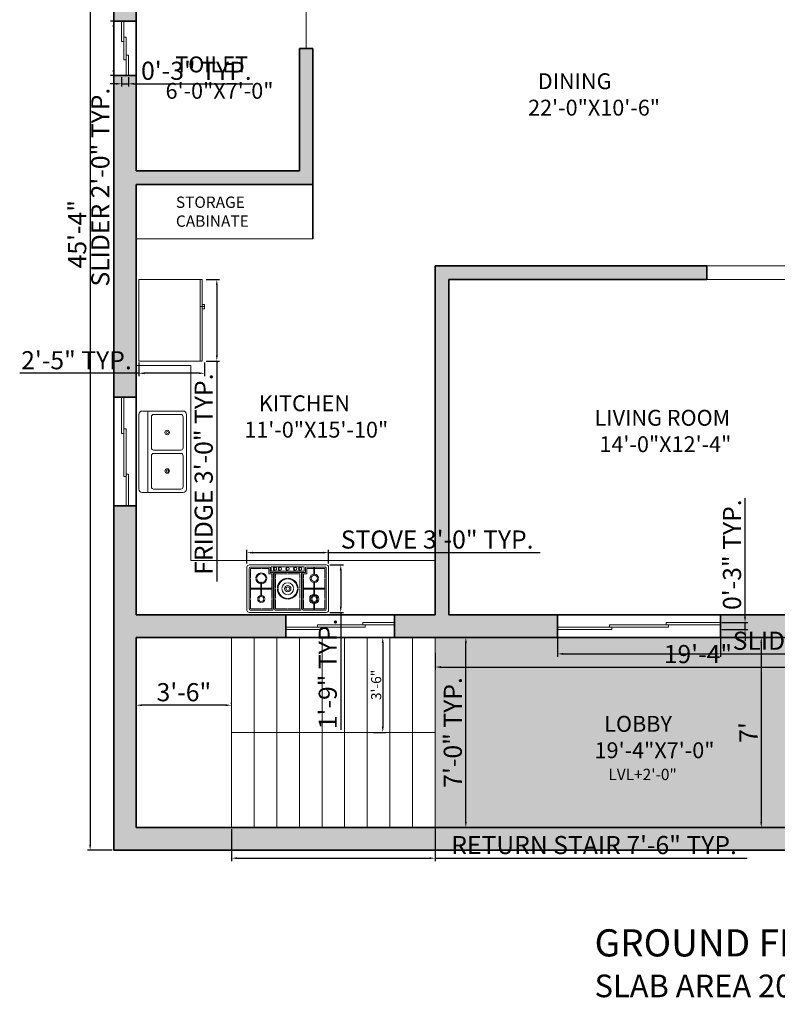
# Model space of a CAD drawing. Units: inches. Extents: x 3491 to 6898, y 1360 to 2019.
# Tile 1 of 9: x 3491 to 3825, y 1360 to 1795. Entities that reach past the tile are written whole.
import ezdxf

# ---------------------------------------------------------------- set-up
doc = ezdxf.new("R2010")
doc.units = ezdxf.units.IN
for name, color, linetype, lineweight in [('A-ANNO-DIMS', 2, 'Continuous', 18), ('A-ANNO-TEXT', 7, 'Continuous', 18), ('A-ANNO-TITL', 7, 'Continuous', 30), ('A-AREA-IDEN', 7, 'Continuous', 18), ('A-DOOR', 4, 'Continuous', 18), ('A-EQPM', 8, 'Continuous', 18), ('A-FLOR-CASE', 8, 'Continuous', 18), ('A-FLOR-FIXT', 8, 'Continuous', 18), ('A-FLOR-PATT', 252, 'Continuous', 13), ('A-FLOR-STRS', 7, 'Continuous', 18), ('A-GLAZ', 5, 'Continuous', 18), ('A-WALL', 7, 'Continuous', 35), ('A-WALL-PATT', 8, 'Continuous', 13)]:
    doc.layers.add(name, color=color, linetype=linetype, lineweight=lineweight)
doc.layers.add('A-WALL-OPEN', color=251, linetype='Continuous', lineweight=13, true_color=0x636466)
doc.styles.get("Standard").update_dxf_attribs({"font": 'arial.ttf'})
doc.dimstyles.new('ISO-25', dxfattribs={"dimtxt": 8, "dimasz": 2.5, "dimexe": 1.25, "dimexo": 0.625, "dimtad": 1, "dimdec": 1, "dimlunit": 3, "dimtxsty": 'Standard', "dimcen": 2.5, "dimclrt": 1, "dimadec": 0, "dimazin": 0, "dimtfac": 1, "dimtdec": 1, "dimtmove": 0, "dimatfit": 3, "dimfxl": 1, "dimarcsym": 0})

# ---------------------------------------------------------------- blocks, each defined once
blk = doc.blocks.new('*D4')
at = {"layer": 'A-ANNO-DIMS', "color": 0, "lineweight": -2, "transparency": 16777216}
for p, q in [((3531.51, 1972.37), (3520.5, 1972.37)), ((3521.75, 1969.87), (3521.75, 1430.87)), ((3531.51, 1428.37), (3520.5, 1428.37))]:
    blk.add_line(p, q, dxfattribs=at)
at = {"layer": 'A-ANNO-DIMS', "color": 0, "transparency": 16777216}
for points in [[(3521.33, 1969.87), (3522.17, 1969.87), (3521.75, 1972.37)], [(3521.33, 1430.87), (3522.17, 1430.87), (3521.75, 1428.37)]]:
    blk.add_solid(points, dxfattribs=at)
at = {"layer": 'Defpoints', "color": 0, "transparency": 16777216}
for p in [(3532.13, 1972.37), (3521.75, 1428.37), (3532.13, 1428.37)]:
    blk.add_point(p, dxfattribs=at)
at = {"layer": 'A-ANNO-DIMS', "color": 0, "transparency": 16777216, "insert": (3517.06, 1700.37), "char_height": 8, "attachment_point": 5, "rotation": 90}
blk.add_mtext('45\'-4"', dxfattribs=at)
blk = doc.blocks.new('*D5')
at = {"layer": 'A-ANNO-DIMS', "color": 0, "lineweight": -2, "transparency": 16777216}
for p, q in [((3542.13, 1493.03), (3542.13, 1493.65)), ((3581.63, 1492.4), (3544.63, 1492.4)), ((3584.13, 1493.03), (3584.13, 1493.65))]:
    blk.add_line(p, q, dxfattribs=at)
at = {"layer": 'A-ANNO-DIMS', "color": 0, "transparency": 16777216}
for points in [[(3544.63, 1492.82), (3544.63, 1491.99), (3542.13, 1492.4)], [(3581.63, 1492.82), (3581.63, 1491.99), (3584.13, 1492.4)]]:
    blk.add_solid(points, dxfattribs=at)
at = {"layer": 'Defpoints', "color": 0, "transparency": 16777216}
for p in [(3542.13, 1492.4), (3542.13, 1492.4), (3584.13, 1492.4)]:
    blk.add_point(p, dxfattribs=at)
at = {"layer": 'A-ANNO-DIMS', "color": 0, "transparency": 16777216, "insert": (3563.13, 1497.12), "char_height": 8, "attachment_point": 5}
blk.add_mtext('3\'-6"', dxfattribs=at)
blk = doc.blocks.new('*D6')
at = {"layer": 'A-ANNO-DIMS', "color": 0, "lineweight": -2, "transparency": 16777216}
for p, q in [((3646.84, 1522.37), (3652.19, 1522.37)), ((3650.94, 1519.87), (3650.94, 1482.87)), ((3646.84, 1480.37), (3652.19, 1480.37))]:
    blk.add_line(p, q, dxfattribs=at)
at = {"layer": 'A-ANNO-DIMS', "color": 0, "transparency": 16777216}
for points in [[(3650.52, 1519.87), (3651.36, 1519.87), (3650.94, 1522.37)], [(3650.52, 1482.87), (3651.36, 1482.87), (3650.94, 1480.37)]]:
    blk.add_solid(points, dxfattribs=at)
at = {"layer": 'Defpoints', "color": 0, "transparency": 16777216}
for p in [(3646.22, 1522.37), (3646.22, 1480.37), (3650.94, 1480.37)]:
    blk.add_point(p, dxfattribs=at)
at = {"layer": 'A-ANNO-DIMS', "color": 0, "transparency": 16777216, "insert": (3648.04, 1501.37), "char_height": 8, "attachment_point": 5, "rotation": 90}
blk.add_mtext('{\\H0.55556x;3\'-6"}', dxfattribs=at)
blk = doc.blocks.new('*D7')
at = {"layer": 'A-ANNO-DIMS', "color": 0, "lineweight": -2, "transparency": 16777216}
for p, q in [((3818.73, 1522.37), (3819.35, 1522.37)), ((3818.1, 1519.87), (3818.1, 1440.87)), ((3818.73, 1438.37), (3819.35, 1438.37))]:
    blk.add_line(p, q, dxfattribs=at)
at = {"layer": 'A-ANNO-DIMS', "color": 0, "transparency": 16777216}
for points in [[(3817.69, 1519.87), (3818.52, 1519.87), (3818.1, 1522.37)], [(3817.69, 1440.87), (3818.52, 1440.87), (3818.1, 1438.37)]]:
    blk.add_solid(points, dxfattribs=at)
at = {"layer": 'Defpoints', "color": 0, "transparency": 16777216}
for p in [(3818.1, 1522.37), (3818.1, 1438.37), (3818.1, 1438.37)]:
    blk.add_point(p, dxfattribs=at)
at = {"layer": 'A-ANNO-DIMS', "color": 0, "transparency": 16777216, "insert": (3813.48, 1480.37), "char_height": 8, "attachment_point": 5, "rotation": 90}
blk.add_mtext("7'", dxfattribs=at)
blk = doc.blocks.new('*D8')
at = {"layer": 'A-ANNO-DIMS', "color": 0, "lineweight": -2, "transparency": 16777216}
for p, q in [((3906.13, 1521.74), (3906.13, 1507.99)), ((3674.13, 1515.52), (3674.13, 1507.99)), ((3676.63, 1509.24), (3903.63, 1509.24))]:
    blk.add_line(p, q, dxfattribs=at)
at = {"layer": 'A-ANNO-DIMS', "color": 0, "transparency": 16777216}
for points in [[(3676.63, 1509.66), (3676.63, 1508.83), (3674.13, 1509.24)], [(3903.63, 1509.66), (3903.63, 1508.83), (3906.13, 1509.24)]]:
    blk.add_solid(points, dxfattribs=at)
at = {"layer": 'Defpoints', "color": 0, "transparency": 16777216}
for p in [(3906.13, 1522.37), (3674.13, 1516.15), (3906.13, 1509.24)]:
    blk.add_point(p, dxfattribs=at)
at = {"layer": 'A-ANNO-DIMS', "color": 0, "transparency": 16777216, "insert": (3790.13, 1513.95), "char_height": 8, "attachment_point": 5}
blk.add_mtext('19\'-4"', dxfattribs=at)
blk = doc.blocks.new('STOVE')
for p, q in [((11.85, 19.7), (11.55, 19.7)), ((11.55, 16.92), (11.55, 19.7)), ((11.85, 16.92), (11.85, 19.7)), ((-11.85, 13.73), (-11.85, 7.62)), ((-11.85, 13.73), (-11.55, 13.73)), ((-11.55, 13.73), (-11.55, 7.62)), ((11.85, 16.92), (11.55, 16.92)), ((11.85, 13.23), (11.55, 13.23)), ((11.55, 13.23), (11.55, 7.57)), ((11.85, 13.23), (11.85, 7.57)), ((-11.85, 10.75), (-16.4, 10.75)), ((-11.85, 10.25), (-16.4, 10.25)), ((-7, 10.75), (-11.55, 10.75)), ((-7, 10.25), (-11.55, 10.25)), ((7, 10.75), (11.55, 10.75)), ((7, 10.25), (11.55, 10.25)), ((11.85, 10.75), (16.4, 10.75)), ((11.85, 10.25), (16.4, 10.25)), ((-11.85, 7.62), (-11.55, 7.62)), ((11.85, 7.57), (11.55, 7.57)), ((-7, 3.9), (-8.4, 3.9)), ((-7.8, 3.3), (-7.8, 1)), ((-6.4, 3.3), (-7.8, 3.3)), ((7.3, 2.8), (-7.3, 2.8)), ((-7.3, 2.8), (-7.3, 0.8)), ((7.3, 0.8), (-7.3, 0.8)), ((-5.4, 3.9), (-6, 3.9)), ((-5.4, 3.9), (-0.15, 3.9)), ((0.15, 3.9), (5.4, 3.9)), ((6.4, 3.3), (7.8, 3.3)), ((7, 3.9), (8.4, 3.9)), ((7.3, 2.8), (7.3, 0.8)), ((7.8, 3.3), (7.8, 1)), ((8.4, 3.9), (8.4, 1.6)), ((11.85, 4.28), (11.55, 4.28)), ((11.55, 4.28), (11.55, 1.3)), ((11.85, 1.3), (11.55, 1.3)), ((11.85, 4.28), (11.85, 1.3))]:
    blk.add_line(p, q)
for points in [[(-17, 21), (17, 21, -0.414214), (18, 20), (18, 1, -0.414214), (17, 0), (-17, 0, -0.414214), (-18, 1), (-18, 20, -0.414214)], [(6, 3.3), (-6, 3.3), (-6, 19.4, -0.414214), (-5.4, 20), (5.4, 20, -0.414214), (6, 19.4)]]:
    blk.add_lwpolyline(points, format="xyb", close=True)
for points in [[(-7.8, 1), (-16.4, 1, -0.414214), (-17, 1.6), (-17, 19.4, -0.414214), (-16.4, 20), (-7, 20, -0.414214), (-6.4, 19.4), (-6.4, 3.3)], [(6.4, 19.4, -0.414214), (7, 20), (16.4, 20, -0.414214), (17, 19.4), (17, 1.6, -0.414214), (16.4, 1), (7.8, 1)]]:
    blk.add_lwpolyline(points, format="xyb")
for points in [[(-16.4, 15.22), (-16.4, 19.4), (-11.85, 19.4)], [(-11.55, 19.4), (-7, 19.4), (-7, 15.22)], [(-5.4, 15.22), (-5.4, 19.4), (-0.15, 19.4)], [(0.15, 19.4), (5.4, 19.4), (5.4, 15.22)], [(6.4, 3.3), (6.4, 19.4)], [(7, 15.22), (7, 19.4), (11.55, 19.4)], [(11.85, 19.4), (16.4, 19.4), (16.4, 15.22)], [(-16.4, 6.08), (-16.4, 14.92)], [(-7, 14.92), (-7, 6.08)], [(-5.4, 10.65), (-5.4, 14.92)], [(5.4, 14.92), (5.4, 10.65)], [(7, 6.08), (7, 14.92)], [(16.4, 14.92), (16.4, 6.08)], [(-5.4, 6.08), (-5.4, 10.35)], [(5.4, 10.35), (5.4, 6.08)], [(-11.85, 1.6), (-16.4, 1.6), (-16.4, 5.77)], [(-7, 5.77), (-7, 3.9)], [(-5.4, 3.9), (-5.4, 5.77)], [(5.4, 5.77), (5.4, 3.9)], [(7, 3.9), (7, 5.77)], [(16.4, 5.77), (16.4, 1.6), (11.85, 1.6)], [(-8.4, 3.9), (-8.4, 1.6), (-11.55, 1.6)], [(11.55, 1.6), (8.4, 1.6)]]:
    blk.add_lwpolyline(points)
for centre, radius in [((-11.7, 15.07), 1.1), ((11.7, 15.07), 1.6), ((11.7, 15.07), 1.1), ((0, 10.5), 1.4), ((0, 10.5), 0.8), ((11.7, 5.93), 1.4), ((-5.49, 1.8), 0.6), ((-3.3, 1.8), 0.6), ((0, 1.8), 0.6), ((3.39, 1.8), 0.6), ((5.57, 1.8), 0.6)]:
    blk.add_circle(centre, radius)
for centre, radius, start, end in [((-11.7, 15.07), 1.6, 95.3794, 174.6206), ((-11.7, 15.07), 1.6, 185.3794, 264.6206), ((-11.7, 15.07), 1.6, 5.3794, 84.6206), ((-11.7, 15.07), 1.6, 275.3794, 354.6206), ((0, 10.5), 4.6, 91.8687, 178.1313), ((0, 10.5), 4.3, 91.9991, 178.0009), ((0, 10.5), 2.6, 93.3074, 176.6926), ((0, 10.5), 4.6, 1.8687, 88.1313), ((0, 10.5), 4.3, 1.9991, 88.0009), ((0, 10.5), 2.6, 3.3074, 86.6926), ((11.7, 15.07), 2.1, 94.096, 175.904), ((11.7, 15.07), 2.1, 184.096, 265.904), ((11.7, 15.07), 2.1, 4.096, 85.904), ((11.7, 15.07), 2.1, 274.096, 355.904), ((0, 10.5), 4.6, 181.8687, 268.1313), ((0, 10.5), 4.3, 181.9991, 268.0009), ((0, 10.5), 2.6, 183.3074, 266.6926), ((0, 10.5), 4.6, 271.8687, 358.1313), ((0, 10.5), 4.3, 271.9991, 358.0009), ((0, 10.5), 2.6, 273.3074, 356.6926), ((-11.7, 5.93), 2.4, 93.5833, 176.4167), ((-11.7, 5.93), 2.4, 183.5833, 266.4167), ((-11.7, 5.93), 2, 94.3012, 175.6988), ((-11.7, 5.93), 2, 184.3012, 265.6988), ((-11.7, 5.93), 2.4, 3.5833, 86.4167), ((-11.7, 5.93), 2, 4.3012, 85.6988), ((-11.7, 5.93), 2.4, 273.5833, 356.4167), ((-11.7, 5.93), 2, 274.3012, 355.6988), ((11.7, 5.93), 1.9, 94.5281, 175.4719), ((11.7, 5.93), 1.9, 184.5281, 265.4719), ((11.7, 5.93), 1.9, 4.5281, 85.4719), ((11.7, 5.93), 1.9, 274.5281, 355.4719), ((-5.49, 1.8), 0.846, 89.9979, 270), ((-3.3, 1.8), 0.846, 89.9979, 270), ((0, 1.8), 0.846, 89.9979, 270), ((3.39, 1.8), 0.846, 89.9979, 270), ((5.57, 1.8), 0.846, 89.9979, 270)]:
    blk.add_arc(centre, radius, start, end)
blk = doc.blocks.new('Sink-double - 36 in top')
for p, q in [((-18, -4), (18, -4)), ((-0.75, -18.5), (-0.75, -6.5)), ((0.75, -6.5), (0.75, -18.5))]:
    blk.add_line(p, q)
for points in [[(-16.5, 0), (16.5, 0)], [(-18, -19.5), (-18, -1.5)], [(18, -1.5), (18, -19.5)], [(-16.5, -18.5), (-16.5, -6.5)], [(-15.5, -5.5), (-1.75, -5.5)], [(1.75, -5.5), (15.5, -5.5)], [(16.5, -6.5), (16.5, -18.5)], [(16.5, -21), (-16.5, -21)], [(-1.75, -19.5), (-15.5, -19.5)], [(15.5, -19.5), (1.75, -19.5)]]:
    blk.add_lwpolyline(points)
for centre, radius in [((-8.5, -12.5), 1), ((-8.5, -12.5), 0.5), ((8.5, -12.5), 1), ((8.5, -12.5), 0.5)]:
    blk.add_circle(centre, radius)
for centre, radius, start, end in [((-16.5, -1.5), 1.5, 90, 180), ((16.5, -1.5), 1.5, 0, 90), ((-15.5, -6.5), 1, 90, 180), ((-1.75, -6.5), 1, 0, 90), ((1.75, -6.5), 1, 90, 180), ((15.5, -6.5), 1, 0, 90), ((-16.5, -19.5), 1.5, 180, 270), ((-15.5, -18.5), 1, 180, 270), ((-1.75, -18.5), 1, 270, 0), ((1.75, -18.5), 1, 180, 270), ((15.5, -18.5), 1, 270, 0), ((16.5, -19.5), 1.5, 270, 0)]:
    blk.add_arc(centre, radius, start, end)
blk = doc.blocks.new('Refrigerator-2 door - 36 in top')
for p, q in [((0, -26.999999), (36, -26.999999)), ((11, -27.999999), (11, -28.999999)), ((11, -28.999999), (13, -28.999999)), ((12, -26.999999), (12, -28.999999)), ((13, -28.999999), (13, -27.999999))]:
    blk.add_line(p, q)
blk.add_lwpolyline([(0, -27.999999), (0, 0), (36, 0), (36, -27.999999)], close=True)
blk = doc.blocks.new('WIN-SLIDER-24IN')
for p, q in [((0, 1), (17, 1)), ((0, 0), (9, 0)), ((7, 1), (7, 2)), ((7, 2), (24, 2)), ((9, 0), (9, 1)), ((15, 2), (15, 3)), ((15, 3), (24, 3)), ((17, 1), (17, 2))]:
    blk.add_line(p, q)
blk = doc.blocks.new('WIN-SLIDER-48IN')
for p, q in [((35, 1), (0, 1)), ((48, 2), (14, 2)), ((14, 2), (14, 1)), ((16, 1), (16, 0)), ((34, 3), (34, 2)), ((48, 3), (34, 3)), ((35, 2), (35, 1)), ((16, 0), (0, 0))]:
    blk.add_line(p, q)
blk = doc.blocks.new('WIN-SLIDER-72IN')
for p, q in [((0, 1), (49, 1)), ((0, 0), (23.95, 0)), ((22.95, 2), (72, 2)), ((22.95, 1), (22.95, 2)), ((23.95, 0), (23.95, 1)), ((48, 3), (72, 3)), ((48, 2), (48, 3)), ((49, 1), (49, 2))]:
    blk.add_line(p, q)
blk = doc.blocks.new('STAIR-RETURN-FLIGHT')
for p, q in [((0, 84), (0, 0)), ((10, 84), (10, 0)), ((20, 84), (20, 0)), ((30, 84), (30, 0)), ((40, 84), (40, 0)), ((50, 84), (50, 0)), ((60, 84), (60, 0)), ((70, 84), (70, 0)), ((80, 84), (80, 0)), ((0, 42), (90, 42))]:
    blk.add_line(p, q)
blk = doc.blocks.new('COUNTER-KITCHEN-L')
for p, q in [((24, 86.04), (0, 86.04)), ((24, 86.04), (24, 0)), ((132, 0), (24, 0))]:
    blk.add_line(p, q)
blk = doc.blocks.new('*D110')
at = {"layer": 'A-ANNO-DIMS', "color": 0, "lineweight": -2, "transparency": 16777216}
for p, q in [((3535.01, 1794.37), (3530.78, 1794.37)), ((3532.03, 1791.87), (3532.03, 1772.87)), ((3535.01, 1770.37), (3530.78, 1770.37)), ((3532.03, 1770.37), (3532.03, 1674.41))]:
    blk.add_line(p, q, dxfattribs=at)
at = {"layer": 'A-ANNO-DIMS', "color": 0, "transparency": 16777216}
for points in [[(3531.62, 1791.87), (3532.45, 1791.87), (3532.03, 1794.37)], [(3531.62, 1772.87), (3532.45, 1772.87), (3532.03, 1770.37)]]:
    blk.add_solid(points, dxfattribs=at)
at = {"layer": 'Defpoints', "color": 0, "transparency": 16777216}
for p in [(3535.63, 1794.37), (3532.03, 1770.37), (3535.63, 1770.37)]:
    blk.add_point(p, dxfattribs=at)
at = {"layer": 'A-ANNO-DIMS', "color": 1, "transparency": 16777216, "insert": (3527.27, 1721.14), "char_height": 8, "attachment_point": 5, "rotation": 90}
blk.add_mtext('SLIDER 2\'-0" TYP.', dxfattribs=at)
blk = doc.blocks.new('*D111')
at = {"layer": 'A-ANNO-DIMS', "color": 0, "lineweight": -2, "transparency": 16777216}
for p, q in [((3535.63, 1769.74), (3535.63, 1765.52)), ((3538.63, 1769.74), (3538.63, 1765.52)), ((3533.13, 1766.77), (3530.63, 1766.77)), ((3535.63, 1766.77), (3538.63, 1766.77)), ((3541.13, 1766.77), (3593.65, 1766.77))]:
    blk.add_line(p, q, dxfattribs=at)
at = {"layer": 'A-ANNO-DIMS', "color": 0, "transparency": 16777216}
for points in [[(3533.13, 1767.18), (3533.13, 1766.35), (3535.63, 1766.77)], [(3541.13, 1767.18), (3541.13, 1766.35), (3538.63, 1766.77)]]:
    blk.add_solid(points, dxfattribs=at)
at = {"layer": 'Defpoints', "color": 0, "transparency": 16777216}
for p in [(3535.63, 1770.37), (3538.63, 1770.37), (3538.63, 1766.77)]:
    blk.add_point(p, dxfattribs=at)
at = {"layer": 'A-ANNO-DIMS', "color": 1, "transparency": 16777216, "insert": (3568.64, 1771.48), "char_height": 8, "attachment_point": 5}
blk.add_mtext('0\'-3" TYP.', dxfattribs=at)
blk = doc.blocks.new('*D120')
at = {"layer": 'A-ANNO-DIMS', "color": 0, "lineweight": -2, "transparency": 16777216}
for p, q in [((3728.13, 1525.24), (3728.13, 1513.82)), ((3800.13, 1525.24), (3800.13, 1513.82)), ((3730.63, 1515.07), (3797.63, 1515.07)), ((3800.13, 1515.07), (3896.08, 1515.07))]:
    blk.add_line(p, q, dxfattribs=at)
at = {"layer": 'A-ANNO-DIMS', "color": 0, "transparency": 16777216}
for points in [[(3730.63, 1515.48), (3730.63, 1514.65), (3728.13, 1515.07)], [(3797.63, 1515.48), (3797.63, 1514.65), (3800.13, 1515.07)]]:
    blk.add_solid(points, dxfattribs=at)
at = {"layer": 'Defpoints', "color": 0, "transparency": 16777216}
for p in [(3728.13, 1525.87), (3800.13, 1525.87), (3800.13, 1515.07)]:
    blk.add_point(p, dxfattribs=at)
at = {"layer": 'A-ANNO-DIMS', "color": 1, "transparency": 16777216, "insert": (3849.36, 1519.83), "char_height": 8, "attachment_point": 5}
blk.add_mtext('SLIDER 6\'-0" TYP.', dxfattribs=at)
blk = doc.blocks.new('*D121')
at = {"layer": 'A-ANNO-DIMS', "color": 0, "lineweight": -2, "transparency": 16777216}
for p, q in [((3810.93, 1531.37), (3810.93, 1583.88)), ((3800.76, 1528.87), (3812.18, 1528.87)), ((3800.76, 1525.87), (3812.18, 1525.87)), ((3810.93, 1525.87), (3810.93, 1528.87)), ((3810.93, 1523.37), (3810.93, 1520.87))]:
    blk.add_line(p, q, dxfattribs=at)
at = {"layer": 'A-ANNO-DIMS', "color": 0, "transparency": 16777216}
for points in [[(3810.52, 1531.37), (3811.35, 1531.37), (3810.93, 1528.87)], [(3810.52, 1523.37), (3811.35, 1523.37), (3810.93, 1525.87)]]:
    blk.add_solid(points, dxfattribs=at)
at = {"layer": 'Defpoints', "color": 0, "transparency": 16777216}
for p in [(3800.13, 1528.87), (3800.13, 1525.87), (3810.93, 1528.87)]:
    blk.add_point(p, dxfattribs=at)
at = {"layer": 'A-ANNO-DIMS', "color": 1, "transparency": 16777216, "insert": (3806.22, 1558.87), "char_height": 8, "attachment_point": 5, "rotation": 90}
blk.add_mtext('0\'-3" TYP.', dxfattribs=at)
blk = doc.blocks.new('*D124')
at = {"layer": 'A-ANNO-DIMS', "color": 0, "lineweight": -2, "transparency": 16777216}
for p, q in [((3591, 1554.99), (3591, 1561.02)), ((3627, 1554.99), (3627, 1561.02)), ((3593.5, 1559.77), (3624.5, 1559.77)), ((3627, 1559.77), (3720.47, 1559.77))]:
    blk.add_line(p, q, dxfattribs=at)
at = {"layer": 'A-ANNO-DIMS', "color": 0, "transparency": 16777216}
for points in [[(3593.5, 1560.18), (3593.5, 1559.35), (3591, 1559.77)], [(3624.5, 1560.18), (3624.5, 1559.35), (3627, 1559.77)]]:
    blk.add_solid(points, dxfattribs=at)
at = {"layer": 'Defpoints', "color": 0, "transparency": 16777216}
for p in [(3627, 1559.77), (3591, 1554.37), (3627, 1554.37)]:
    blk.add_point(p, dxfattribs=at)
at = {"layer": 'A-ANNO-DIMS', "color": 1, "transparency": 16777216, "insert": (3674.98, 1564.53), "char_height": 8, "attachment_point": 5}
blk.add_mtext('STOVE 3\'-0" TYP.', dxfattribs=at)
blk = doc.blocks.new('*D125')
at = {"layer": 'A-ANNO-DIMS', "color": 0, "lineweight": -2, "transparency": 16777216}
for p, q in [((3627.63, 1554.37), (3633.65, 1554.37)), ((3632.4, 1551.87), (3632.4, 1535.87)), ((3627.63, 1533.37), (3633.65, 1533.37)), ((3632.4, 1533.37), (3632.4, 1481.6))]:
    blk.add_line(p, q, dxfattribs=at)
at = {"layer": 'A-ANNO-DIMS', "color": 0, "transparency": 16777216}
for points in [[(3631.99, 1551.87), (3632.82, 1551.87), (3632.4, 1554.37)], [(3631.99, 1535.87), (3632.82, 1535.87), (3632.4, 1533.37)]]:
    blk.add_solid(points, dxfattribs=at)
at = {"layer": 'Defpoints', "color": 0, "transparency": 16777216}
for p in [(3627, 1554.37), (3627, 1533.37), (3632.4, 1533.37)]:
    blk.add_point(p, dxfattribs=at)
at = {"layer": 'A-ANNO-DIMS', "color": 1, "transparency": 16777216, "insert": (3627.69, 1506.24), "char_height": 8, "attachment_point": 5, "rotation": 90}
blk.add_mtext('1\'-9" TYP.', dxfattribs=at)
blk = doc.blocks.new('*D128')
at = {"layer": 'A-ANNO-DIMS', "color": 0, "lineweight": -2, "transparency": 16777216}
for p, q in [((3572.9, 1680.37), (3578.93, 1680.37)), ((3577.68, 1677.87), (3577.68, 1646.87)), ((3572.9, 1644.37), (3578.93, 1644.37)), ((3577.68, 1644.37), (3577.68, 1546.98))]:
    blk.add_line(p, q, dxfattribs=at)
at = {"layer": 'A-ANNO-DIMS', "color": 0, "transparency": 16777216}
for points in [[(3577.26, 1677.87), (3578.09, 1677.87), (3577.68, 1680.37)], [(3577.26, 1646.87), (3578.09, 1646.87), (3577.68, 1644.37)]]:
    blk.add_solid(points, dxfattribs=at)
at = {"layer": 'Defpoints', "color": 0, "transparency": 16777216}
for p in [(3572.28, 1680.37), (3572.28, 1644.37), (3577.68, 1644.37)]:
    blk.add_point(p, dxfattribs=at)
at = {"layer": 'A-ANNO-DIMS', "color": 1, "transparency": 16777216, "insert": (3572.91, 1594.42), "char_height": 8, "attachment_point": 5, "rotation": 90}
blk.add_mtext('FRIDGE 3\'-0" TYP.', dxfattribs=at)
blk = doc.blocks.new('*D129')
at = {"layer": 'A-ANNO-DIMS', "color": 0, "lineweight": -2, "transparency": 16777216}
for p, q in [((3543.28, 1643.74), (3543.28, 1637.72)), ((3572.28, 1643.74), (3572.28, 1637.72)), ((3543.28, 1638.97), (3490.63, 1638.97)), ((3569.78, 1638.97), (3545.78, 1638.97))]:
    blk.add_line(p, q, dxfattribs=at)
at = {"layer": 'A-ANNO-DIMS', "color": 0, "transparency": 16777216}
for points in [[(3545.78, 1639.38), (3545.78, 1638.55), (3543.28, 1638.97)], [(3569.78, 1639.38), (3569.78, 1638.55), (3572.28, 1638.97)]]:
    blk.add_solid(points, dxfattribs=at)
at = {"layer": 'Defpoints', "color": 0, "transparency": 16777216}
for p in [(3543.28, 1644.37), (3572.28, 1644.37), (3543.28, 1638.97)]:
    blk.add_point(p, dxfattribs=at)
at = {"layer": 'A-ANNO-DIMS', "color": 1, "transparency": 16777216, "insert": (3515.7, 1643.68), "char_height": 8, "attachment_point": 5}
blk.add_mtext('2\'-5" TYP.', dxfattribs=at)
blk = doc.blocks.new('*D130')
at = {"layer": 'A-ANNO-DIMS', "color": 0, "lineweight": -2, "transparency": 16777216}
for p, q in [((3584.13, 1437.74), (3584.13, 1423.62)), ((3674.13, 1437.74), (3674.13, 1423.62)), ((3586.63, 1424.87), (3671.63, 1424.87)), ((3674.13, 1424.87), (3811.92, 1424.87))]:
    blk.add_line(p, q, dxfattribs=at)
at = {"layer": 'A-ANNO-DIMS', "color": 0, "transparency": 16777216}
for points in [[(3586.63, 1425.28), (3586.63, 1424.45), (3584.13, 1424.87)], [(3671.63, 1425.28), (3671.63, 1424.45), (3674.13, 1424.87)]]:
    blk.add_solid(points, dxfattribs=at)
at = {"layer": 'Defpoints', "color": 0, "transparency": 16777216}
for p in [(3584.13, 1438.37), (3674.13, 1438.37), (3674.13, 1424.87)]:
    blk.add_point(p, dxfattribs=at)
at = {"layer": 'A-ANNO-DIMS', "color": 1, "transparency": 16777216, "insert": (3744.28, 1429.63), "char_height": 8, "attachment_point": 5}
blk.add_mtext('RETURN STAIR 7\'-6" TYP.', dxfattribs=at)
blk = doc.blocks.new('*D131')
at = {"layer": 'A-ANNO-DIMS', "color": 0, "lineweight": -2, "transparency": 16777216}
for p, q in [((3674.76, 1522.37), (3688.88, 1522.37)), ((3687.63, 1440.87), (3687.63, 1519.87)), ((3674.76, 1438.37), (3688.88, 1438.37))]:
    blk.add_line(p, q, dxfattribs=at)
at = {"layer": 'A-ANNO-DIMS', "color": 0, "transparency": 16777216}
for points in [[(3687.22, 1519.87), (3688.05, 1519.87), (3687.63, 1522.37)], [(3687.22, 1440.87), (3688.05, 1440.87), (3687.63, 1438.37)]]:
    blk.add_solid(points, dxfattribs=at)
at = {"layer": 'Defpoints', "color": 0, "transparency": 16777216}
for p in [(3674.13, 1522.37), (3687.63, 1522.37), (3674.13, 1438.37)]:
    blk.add_point(p, dxfattribs=at)
at = {"layer": 'A-ANNO-DIMS', "color": 1, "transparency": 16777216, "insert": (3682.92, 1480.37), "char_height": 8, "attachment_point": 5, "rotation": 90}
blk.add_mtext('7\'-0" TYP.', dxfattribs=at)

msp = doc.modelspace()

# ---------------------------------------------------------------- hatches: boundary and pattern name
at = {"layer": 'A-FLOR-PATT'}
h = msp.add_hatch(dxfattribs=at)
h.set_pattern_fill('ANSI36', color=256, scale=0.5, angle=45)
h.paths.add_polyline_path([(3674.13, 1438.37), (3906.13, 1438.37), (3906.13, 1522.37), (3674.13, 1522.37)])
h.paths.add_polyline_path([(3821.85, 1474.19), (3821.85, 1486.54), (3805.36, 1486.54), (3805.36, 1474.19)], flags=24)
h.paths.add_polyline_path([(3773.55, 1505.64), (3806.02, 1505.64), (3806.02, 1522.12), (3773.55, 1522.12)], flags=24)
h.paths.add_polyline_path([(3741.67, 1455.94), (3796.08, 1455.94), (3796.08, 1491.16), (3741.67, 1491.16)], flags=24)
at = {"layer": 'A-WALL-PATT'}
h = msp.add_hatch(color=256, dxfattribs=at)
h.dxf.hatch_style = 1
h.paths.add_polyline_path([(3856.13, 1532.37), (3800.13, 1532.37), (3800.13, 1522.37), (3856.13, 1522.37)])
h.paths.add_polyline_path([(3906.13, 1626.37), (3896.13, 1626.37), (3896.13, 1592.37), (3906.13, 1592.37)])
h.paths.add_polyline_path([(3906.13, 1556.37), (3896.13, 1556.37), (3896.13, 1532.37), (3892.13, 1532.37), (3892.13, 1522.37), (3906.13, 1522.37)])
h.paths.add_polyline_path([(3728.13, 1532.37), (3680.13, 1532.37), (3680.13, 1680.37), (3794.13, 1680.37), (3794.13, 1686.37), (3674.13, 1686.37), (3674.13, 1532.37), (3656.16, 1532.37), (3656.16, 1522.37), (3728.13, 1522.37)])
h.paths.add_polyline_path([(3608.16, 1532.37), (3542.13, 1532.37), (3542.13, 1580.4), (3532.13, 1580.4), (3532.13, 1428.37), (3674.13, 1428.37), (3674.13, 1438.37), (3542.13, 1438.37), (3542.13, 1522.37), (3608.16, 1522.37)])
h.paths.add_polyline_path([(3542.13, 1722.37), (3620.13, 1722.37), (3620.13, 1782.37), (3614.13, 1782.37), (3614.13, 1728.37), (3542.13, 1728.37), (3542.13, 1770.37), (3532.13, 1770.37), (3532.13, 1628.4), (3542.13, 1628.4)])
h.paths.add_polyline_path([(3906.13, 1680.37), (3930.13, 1680.37), (3930.13, 1686.37), (3890.13, 1686.37), (3890.13, 1776.37), (3884.13, 1776.37), (3884.13, 1686.37), (3872.13, 1686.37), (3872.13, 1680.37), (3896.13, 1680.37), (3896.13, 1668.37), (3906.13, 1668.37)])
h.paths.add_polyline_path([(4054.13, 1719.37), (4044.13, 1719.37), (4044.13, 1686.37), (3978.13, 1686.37), (3978.13, 1680.37), (4054.13, 1680.37)])
h.paths.add_polyline_path([(4054.13, 1857.37), (4044.13, 1857.37), (4044.13, 1818.37), (3884.13, 1818.37), (3884.13, 1812.37), (4044.13, 1812.37), (4044.13, 1779.37), (4054.13, 1779.37)])
h.paths.add_polyline_path([(3848.13, 1872.37), (3842.13, 1872.37), (3842.13, 1818.37), (3782.13, 1818.37), (3782.13, 1902.37), (3800.13, 1902.37), (3800.13, 1908.37), (3758.13, 1908.37), (3758.13, 1902.37), (3776.13, 1902.37), (3776.13, 1818.37), (3716.13, 1818.37), (3716.13, 1872.37), (3710.13, 1872.37), (3710.13, 1812.37), (3848.13, 1812.37)])
h.paths.add_polyline_path([(3542.13, 1857.37), (3532.13, 1857.37), (3532.13, 1794.37), (3542.13, 1794.37), (3542.13, 1812.37), (3674.13, 1812.37), (3674.13, 1818.37), (3542.13, 1818.37)])
h.paths.add_polyline_path([(3542.13, 1962.37), (3710.13, 1962.37), (3710.13, 1938.37), (3716.13, 1938.37), (3716.13, 1962.37), (3842.13, 1962.37), (3842.13, 1938.37), (3848.13, 1938.37), (3848.13, 1962.37), (4044.13, 1962.37), (4044.13, 1923.37), (4054.13, 1923.37), (4054.13, 1972.37), (3532.13, 1972.37), (3532.13, 1923.37), (3542.13, 1923.37)])
h.paths.add_polyline_path([(3734.13, 1908.37), (3710.13, 1908.37), (3710.13, 1902.37), (3734.13, 1902.37)])
h.paths.add_polyline_path([(3848.13, 1908.37), (3824.13, 1908.37), (3824.13, 1902.37), (3848.13, 1902.37)], flags=17)
h = msp.add_hatch(color=256, dxfattribs=at)
h.dxf.hatch_style = 1
h.paths.add_polyline_path([(3918.13, 1438.37), (3674.13, 1438.37), (3674.13, 1428.37), (3918.13, 1428.37)])
h.paths.add_polyline_path([(4072.13, 1621.37), (4054.13, 1621.37), (4054.13, 1680.37), (4044.13, 1680.37), (4044.13, 1615.37), (4066.13, 1615.37), (4066.13, 1438.37), (4038.13, 1438.37), (4038.13, 1428.37), (4072.13, 1428.37)])

# ---------------------------------------------------------------- linework, layer by layer
at = {"layer": 'A-DOOR'}
msp.add_line((3617.13, 1782.37), (3617.13, 1812.37), dxfattribs=at)
at = {"layer": 'A-FLOR-CASE'}
msp.add_line((3620.13, 1698.37), (3542.13, 1698.37), dxfattribs=at)
at = {"layer": 'A-FLOR-STRS'}
msp.add_line((3674.13, 1522.37), (3674.13, 1428.37), dxfattribs=at)
at = {"layer": 'A-WALL'}
for p, q in [((3532.13, 1972.37), (3532.13, 1428.37)), ((3542.13, 1812.37), (3542.13, 1728.37)), ((3542.13, 1794.37), (3532.13, 1794.37)), ((3614.13, 1782.37), (3614.13, 1728.37)), ((3620.13, 1782.37), (3614.13, 1782.37)), ((3620.13, 1782.37), (3620.13, 1698.37)), ((3542.13, 1770.37), (3532.13, 1770.37)), ((3614.13, 1728.37), (3542.13, 1728.37)), ((3620.13, 1722.37), (3542.13, 1722.37)), ((3542.13, 1722.37), (3542.13, 1532.37)), ((3674.13, 1686.37), (3674.13, 1532.37)), ((3794.13, 1686.37), (3674.13, 1686.37)), ((3794.13, 1686.37), (3794.13, 1680.37)), ((3680.13, 1680.37), (3680.13, 1532.37)), ((3794.13, 1680.37), (3680.13, 1680.37)), ((3542.13, 1628.4), (3532.13, 1628.4)), ((3542.13, 1580.4), (3532.13, 1580.4)), ((3674.13, 1532.37), (3542.13, 1532.37)), ((3608.16, 1532.37), (3608.16, 1522.37)), ((3656.16, 1532.37), (3656.16, 1522.37)), ((3896.13, 1532.37), (3680.13, 1532.37)), ((3728.13, 1522.37), (3728.13, 1532.37)), ((3800.13, 1522.37), (3800.13, 1532.37)), ((3906.13, 1522.37), (3542.13, 1522.37)), ((3542.13, 1522.37), (3542.13, 1438.37)), ((3542.13, 1438.37), (3918.13, 1438.37)), ((3532.13, 1428.37), (4072.13, 1428.37))]:
    msp.add_line(p, q, dxfattribs=at)
at = {"layer": 'A-WALL-OPEN'}
for p, q in [((3872.13, 1686.37), (3794.13, 1686.37)), ((3794.13, 1680.37), (3872.13, 1680.37))]:
    msp.add_line(p, q, dxfattribs=at)

# ---------------------------------------------------------------- block references
at = {"layer": 'A-EQPM', "xscale": -1}
for name, p, rotation in [('Refrigerator-2 door - 36 in top', (3543.28, 1680.37), 90), ('STOVE', (3609, 1554.37), 180)]:
    msp.add_blockref(name, p, dxfattribs=dict(at, rotation=rotation))
at = {"layer": 'A-FLOR-CASE'}
msp.add_blockref('COUNTER-KITCHEN-L', (3542.13, 1556.37), dxfattribs=at)
at = {"layer": 'A-FLOR-FIXT', "rotation": 90}
msp.add_blockref('Sink-double - 36 in top', (3543.28, 1604.3), dxfattribs=at)
at = {"layer": 'A-FLOR-STRS'}
msp.add_blockref('STAIR-RETURN-FLIGHT', (3584.13, 1438.37), dxfattribs=at)
at = {"layer": 'A-GLAZ', "rotation": 270}
for name, p in [('WIN-SLIDER-24IN', (3535.63, 1794.37)), ('WIN-SLIDER-48IN', (3535.63, 1628.4))]:
    msp.add_blockref(name, p, dxfattribs=at)
at = {"layer": 'A-GLAZ'}
for name, p in [('WIN-SLIDER-48IN', (3608.16, 1525.87)), ('WIN-SLIDER-72IN', (3728.13, 1525.87))]:
    msp.add_blockref(name, p, dxfattribs=at)

# ---------------------------------------------------------------- texts
at = {"layer": 'A-ANNO-TEXT', "insert": (3559.62, 1716.98), "char_height": 5, "attachment_point": 1}
msp.add_mtext_dynamic_manual_height_columns('STORAGE\\PCABINATE', width=86.9528, gutter_width=12.5, heights=[0], dxfattribs=at)
at = {"layer": 'A-ANNO-TITL', "insert": (3744.49, 1393.48), "char_height": 12, "attachment_point": 1}
msp.add_mtext_dynamic_manual_height_columns('GROUND FLOOR PLAN\\P{\\H0.83333x;SLAB AREA 2004.25sqft}', width=285.9409, gutter_width=12.5, heights=[0], dxfattribs=at)
at = {"layer": 'A-AREA-IDEN', "char_height": 7, "attachment_point": 1}
for s, width, heights, insert in [('  TOILET\\P6\'-0"X7\'-0"', 121.6144, [0], (3555.04, 1778.82)), ('  DINING\\P22\'-0"X10\'-6"', 121.6144, [18.93], (3715.14, 1771.4)), ('   KITCHEN\\P11\'-0"X15\'-10"', 86.9528, [0], (3589.8, 1629.22)), ('LIVING ROOM\\P 14\'-0"X12\'-4"', 121.6144, [0], (3744.49, 1622.81)), ('  LOBBY\\P19\'-4"X7\'-0"\\P{\\H0.71429x;    LVL+2\'-0"}', 121.6144, [0], (3744.49, 1487.68))]:
    msp.add_mtext_dynamic_manual_height_columns(s, width=width, gutter_width=12.5, heights=heights, dxfattribs=dict(at, insert=insert))

# ---------------------------------------------------------------- dimensions: what is measured, and where the dimension line sits
at = {"layer": 'A-ANNO-DIMS'}
for base, p1, p2, picture, middle in [((3521.75, 1428.37), (3532.13, 1972.37), (3532.13, 1428.37), '*D4', (3517.06, 1700.37)), ((3818.1, 1438.37), (3818.1, 1522.37), (3818.1, 1438.37), '*D7', (3813.48, 1480.37))]:
    dim = msp.add_linear_dim(base=base, p1=p1, p2=p2, angle=90, dimstyle='ISO-25', override={"dimclrd": 0, "dimclre": 0, "dimclrt": 0}, dxfattribs=at)
    dim.commit()
    dim.dimension.update_dxf_attribs({"geometry": picture, "text_midpoint": middle})
for base, p1, p2, angle, text, override, picture, middle in [((3532.03, 1770.37), (3535.63, 1794.37), (3535.63, 1770.37), 270, 'SLIDER <> TYP.', {"dimdec": 1, "dimlfac": 1, "dimrnd": 0, "dimzin": 1, "dimdsep": 46, "dimlunit": 4, "dimfrac": 2}, '*D110', (3527.27, 1721.14)), ((3577.68, 1644.37), (3572.28, 1680.37), (3572.28, 1644.37), 270, 'FRIDGE <> TYP.', {"dimdec": 1, "dimlfac": 1, "dimrnd": 0, "dimzin": 1, "dimdsep": 46, "dimlunit": 4, "dimfrac": 2}, '*D128', (3572.91, 1594.42)), ((3543.28, 1638.97), (3572.28, 1644.37), (3543.28, 1644.37), 180, '<> TYP.', {"dimdec": 1, "dimlfac": 1, "dimrnd": 0, "dimzin": 1, "dimdsep": 46, "dimlunit": 4, "dimfrac": 2}, '*D129', (3515.7, 1643.68)), ((3810.93, 1528.87), (3800.13, 1525.87), (3800.13, 1528.87), 90, '<> TYP.', {"dimdec": 1, "dimlfac": 1, "dimrnd": 0, "dimzin": 1, "dimdsep": 46, "dimlunit": 4, "dimfrac": 2}, '*D121', (3806.22, 1558.87)), ((3632.4, 1533.37), (3627, 1554.37), (3627, 1533.37), 270, '<> TYP.', {"dimdec": 1, "dimlfac": 1, "dimrnd": 0, "dimzin": 1, "dimdsep": 46, "dimlunit": 4, "dimfrac": 2}, '*D125', (3627.69, 1506.24)), ((3650.94, 1480.37), (3646.22, 1522.37), (3646.22, 1480.37), 90, '{\\H0.55556x;<>}', {"dimclrd": 0, "dimclre": 0, "dimclrt": 0}, '*D6', (3648.04, 1501.37)), ((3687.63, 1522.37), (3674.13, 1438.37), (3674.13, 1522.37), 90, '<> TYP.', {"dimdec": 1, "dimlfac": 1, "dimrnd": 0, "dimzin": 1, "dimdsep": 46, "dimlunit": 4, "dimfrac": 2}, '*D131', (3682.92, 1480.37))]:
    dim = msp.add_linear_dim(base=base, p1=p1, p2=p2, angle=angle, text=text, dimstyle='ISO-25', override=override, dxfattribs=at)
    dim.commit()
    dim.dimension.update_dxf_attribs({"geometry": picture, "text_midpoint": middle})
for base, p1, p2, text, picture, middle in [((3538.63, 1766.77), (3535.63, 1770.37), (3538.63, 1770.37), '<> TYP.', '*D111', (3568.64, 1771.48)), ((3627, 1559.77), (3591, 1554.37), (3627, 1554.37), 'STOVE <> TYP.', '*D124', (3674.98, 1564.53)), ((3800.13, 1515.07), (3728.13, 1525.87), (3800.13, 1525.87), 'SLIDER <> TYP.', '*D120', (3849.36, 1519.83)), ((3674.13, 1424.87), (3584.13, 1438.37), (3674.13, 1438.37), 'RETURN STAIR <> TYP.', '*D130', (3744.28, 1429.63))]:
    dim = msp.add_linear_dim(base=base, p1=p1, p2=p2, text=text, dimstyle='ISO-25', override={"dimdec": 1, "dimlfac": 1, "dimrnd": 0, "dimzin": 1, "dimdsep": 46, "dimlunit": 4, "dimfrac": 2}, dxfattribs=at)
    dim.commit()
    dim.dimension.update_dxf_attribs({"geometry": picture, "text_midpoint": middle})
for base, p1, p2, picture, middle in [((3906.13, 1509.24), (3674.13, 1516.15), (3906.13, 1522.37), '*D8', (3790.13, 1513.95)), ((3542.13, 1492.4), (3584.13, 1492.4), (3542.13, 1492.4), '*D5', (3563.13, 1497.12))]:
    dim = msp.add_linear_dim(base=base, p1=p1, p2=p2, dimstyle='ISO-25', override={"dimclrd": 0, "dimclre": 0, "dimclrt": 0}, dxfattribs=at)
    dim.commit()
    dim.dimension.update_dxf_attribs({"geometry": picture, "text_midpoint": middle})

doc.saveas('drawing.dxf')
